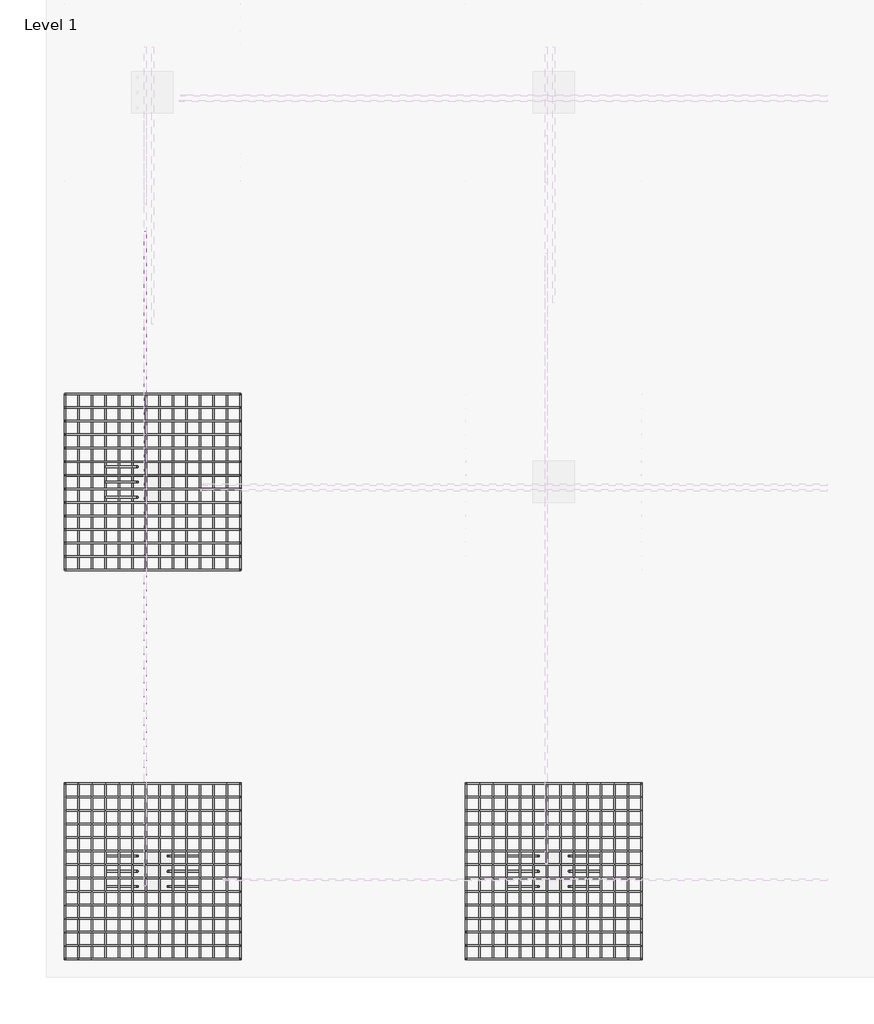
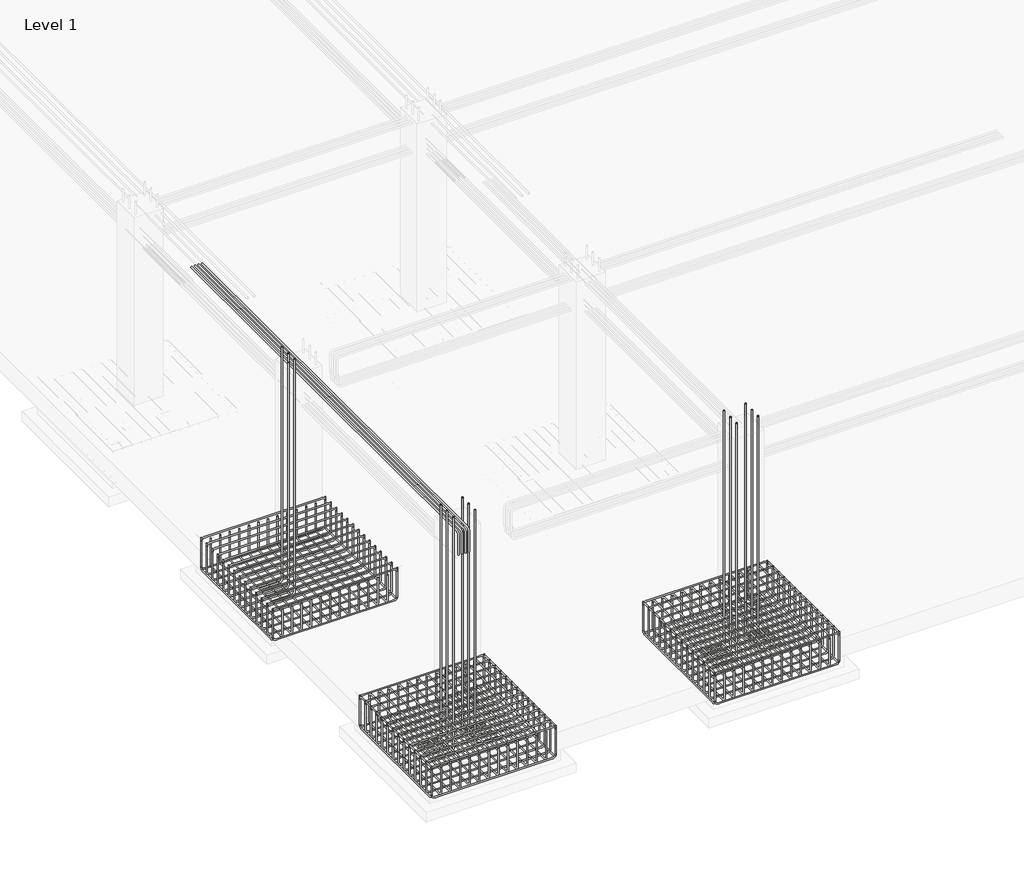
# One storey, part 3 of 17: 18 reinforcing bars.
"""IFC4 building model written with IfcOpenShell, lengths in millimetres."""

from ifc_helpers import new_model, si_unit, point, frame, origin, place, context, project, spatial, polyline, circle_curve, trimmed, segment, composite_curve, source, transform, mapped, element, save
from ifc_brep_helpers import swept_disk

model = new_model("IFC4")

# Units and contexts
model_context = context("Model", 3, world=origin())
ifc_project = project(units=[si_unit("LENGTHUNIT", "METRE", prefix="MILLI")], contexts=[model_context])

# Site, building, storey
site = spatial("IfcSite", under=ifc_project)
building = spatial("IfcBuilding", under=site)
storey = spatial("IfcBuildingStorey", under=building, Name="Level 1", Elevation=0.0)

# Reinforcing bars
placement = place(None, origin())
reinforcing_bar_shape = source(origin(), model_context, "Body", "SolidModel", [
    swept_disk(composite_curve([segment(polyline([(-13686.3632003, 636.009457, -40.0), (-13686.3632003, 636.009457, -504.0)]), True, "CONTINUOUS"), segment(trimmed(circle_curve(frame((-13638.3632003, 636.009457, -504.0), z_axis=(0.0, -1.0, 0.0), x_axis=(-48.0, 0.0, 0.0)), 48.0), [point((-13686.3632003, 636.009457, -504.0))], [point((-13638.3632003, 636.009457, -552.0))], True, "CARTESIAN"), True, "CONTINUOUS"), segment(polyline([(-13638.3632003, 636.009457, -552.0), (-11830.3632003, 636.009457, -552.0)]), True, "CONTINUOUS"), segment(trimmed(circle_curve(frame((-11830.3632003, 636.009457, -504.0), z_axis=(0.0, -1.0, 0.0), x_axis=(0.0, 0.0, -48.0)), 48.0), [point((-11830.3632003, 636.009457, -552.0))], [point((-11782.3632003, 636.009457, -504.0))], True, "CARTESIAN"), True, "CONTINUOUS"), segment(polyline([(-11782.3632003, 636.009457, -504.0), (-11782.3632003, 636.009457, -40.0)]), True, "CONTINUOUS")], self_intersect=False), 8.0),
])
element("IfcReinforcingBar", 1, at=placement, inside=storey, context=model_context, shape_type="MappedRepresentation", body=[
    mapped(reinforcing_bar_shape, transform((0.0, 0.0, 0.0), x_axis=(1.0, 0.0, 0.0), y_axis=(0.0, 1.0, 0.0), z_axis=(0.0, 0.0, 1.0))),
    mapped(reinforcing_bar_shape, transform((0.0, -146.4615385, 0.0), x_axis=(1.0, 0.0, 0.0), y_axis=(0.0, 1.0, 0.0), z_axis=(0.0, 0.0, 1.0))),
    mapped(reinforcing_bar_shape, transform((0.0, -292.9230769, 0.0), x_axis=(1.0, 0.0, 0.0), y_axis=(0.0, 1.0, 0.0), z_axis=(0.0, 0.0, 1.0))),
    mapped(reinforcing_bar_shape, transform((0.0, -439.3846154, 0.0), x_axis=(1.0, 0.0, 0.0), y_axis=(0.0, 1.0, 0.0), z_axis=(0.0, 0.0, 1.0))),
    mapped(reinforcing_bar_shape, transform((0.0, -585.8461538, 0.0), x_axis=(1.0, 0.0, 0.0), y_axis=(0.0, 1.0, 0.0), z_axis=(0.0, 0.0, 1.0))),
    mapped(reinforcing_bar_shape, transform((0.0, -732.3076923, 0.0), x_axis=(1.0, 0.0, 0.0), y_axis=(0.0, 1.0, 0.0), z_axis=(0.0, 0.0, 1.0))),
    mapped(reinforcing_bar_shape, transform((0.0, -878.7692308, 0.0), x_axis=(1.0, 0.0, 0.0), y_axis=(0.0, 1.0, 0.0), z_axis=(0.0, 0.0, 1.0))),
    mapped(reinforcing_bar_shape, transform((0.0, -1025.2307692, 0.0), x_axis=(1.0, 0.0, 0.0), y_axis=(0.0, 1.0, 0.0), z_axis=(0.0, 0.0, 1.0))),
    mapped(reinforcing_bar_shape, transform((0.0, -1171.6923077, 0.0), x_axis=(1.0, 0.0, 0.0), y_axis=(0.0, 1.0, 0.0), z_axis=(0.0, 0.0, 1.0))),
    mapped(reinforcing_bar_shape, transform((0.0, -1318.1538462, 0.0), x_axis=(1.0, 0.0, 0.0), y_axis=(0.0, 1.0, 0.0), z_axis=(0.0, 0.0, 1.0))),
    mapped(reinforcing_bar_shape, transform((0.0, -1464.6153846, 0.0), x_axis=(1.0, 0.0, 0.0), y_axis=(0.0, 1.0, 0.0), z_axis=(0.0, 0.0, 1.0))),
    mapped(reinforcing_bar_shape, transform((0.0, -1611.0769231, 0.0), x_axis=(1.0, 0.0, 0.0), y_axis=(0.0, 1.0, 0.0), z_axis=(0.0, 0.0, 1.0))),
    mapped(reinforcing_bar_shape, transform((0.0, -1757.5384615, 0.0), x_axis=(1.0, 0.0, 0.0), y_axis=(0.0, 1.0, 0.0), z_axis=(0.0, 0.0, 1.0))),
    mapped(reinforcing_bar_shape, transform((0.0, -1904.0, 0.0), x_axis=(1.0, 0.0, 0.0), y_axis=(0.0, 1.0, 0.0), z_axis=(0.0, 0.0, 1.0))),
])
reinforcing_bar_2_shape = source(origin(), model_context, "Body", "SolidModel", [
    swept_disk(composite_curve([segment(polyline([(-13686.3632003, -1267.990543, -504.0), (-13686.3632003, -1267.990543, -96.0)]), True, "CONTINUOUS"), segment(trimmed(circle_curve(frame((-13638.3632003, -1267.990543, -96.0), z_axis=(0.0, 1.0, 0.0), x_axis=(-48.0, 0.0, 0.0)), 48.0), [point((-13686.3632003, -1267.990543, -96.0))], [point((-13638.3632003, -1267.990543, -48.0))], True, "CARTESIAN"), True, "CONTINUOUS"), segment(polyline([(-13638.3632003, -1267.990543, -48.0), (-11830.3632003, -1267.990543, -48.0)]), True, "CONTINUOUS"), segment(trimmed(circle_curve(frame((-11830.3632003, -1267.990543, -96.0), z_axis=(0.0, 1.0, 0.0), x_axis=(0.0, 0.0, 48.0)), 48.0), [point((-11830.3632003, -1267.990543, -48.0))], [point((-11782.3632003, -1267.990543, -96.0))], True, "CARTESIAN"), True, "CONTINUOUS"), segment(polyline([(-11782.3632003, -1267.990543, -96.0), (-11782.3632003, -1267.990543, -504.0)]), True, "CONTINUOUS")], self_intersect=False), 8.0),
])
element("IfcReinforcingBar", 2, at=placement, inside=storey, context=model_context, shape_type="MappedRepresentation", body=[
    mapped(reinforcing_bar_2_shape, transform((0.0, 0.0, 0.0), x_axis=(1.0, 0.0, 0.0), y_axis=(0.0, 1.0, 0.0), z_axis=(0.0, 0.0, 1.0))),
    mapped(reinforcing_bar_2_shape, transform((0.0, 146.4615385, 0.0), x_axis=(1.0, 0.0, 0.0), y_axis=(0.0, 1.0, 0.0), z_axis=(0.0, 0.0, 1.0))),
    mapped(reinforcing_bar_2_shape, transform((0.0, 292.9230769, 0.0), x_axis=(1.0, 0.0, 0.0), y_axis=(0.0, 1.0, 0.0), z_axis=(0.0, 0.0, 1.0))),
    mapped(reinforcing_bar_2_shape, transform((0.0, 439.3846154, 0.0), x_axis=(1.0, 0.0, 0.0), y_axis=(0.0, 1.0, 0.0), z_axis=(0.0, 0.0, 1.0))),
    mapped(reinforcing_bar_2_shape, transform((0.0, 585.8461538, 0.0), x_axis=(1.0, 0.0, 0.0), y_axis=(0.0, 1.0, 0.0), z_axis=(0.0, 0.0, 1.0))),
    mapped(reinforcing_bar_2_shape, transform((0.0, 732.3076923, 0.0), x_axis=(1.0, 0.0, 0.0), y_axis=(0.0, 1.0, 0.0), z_axis=(0.0, 0.0, 1.0))),
    mapped(reinforcing_bar_2_shape, transform((0.0, 878.7692308, 0.0), x_axis=(1.0, 0.0, 0.0), y_axis=(0.0, 1.0, 0.0), z_axis=(0.0, 0.0, 1.0))),
    mapped(reinforcing_bar_2_shape, transform((0.0, 1025.2307692, 0.0), x_axis=(1.0, 0.0, 0.0), y_axis=(0.0, 1.0, 0.0), z_axis=(0.0, 0.0, 1.0))),
    mapped(reinforcing_bar_2_shape, transform((0.0, 1171.6923077, 0.0), x_axis=(1.0, 0.0, 0.0), y_axis=(0.0, 1.0, 0.0), z_axis=(0.0, 0.0, 1.0))),
    mapped(reinforcing_bar_2_shape, transform((0.0, 1318.1538462, 0.0), x_axis=(1.0, 0.0, 0.0), y_axis=(0.0, 1.0, 0.0), z_axis=(0.0, 0.0, 1.0))),
    mapped(reinforcing_bar_2_shape, transform((0.0, 1464.6153846, 0.0), x_axis=(1.0, 0.0, 0.0), y_axis=(0.0, 1.0, 0.0), z_axis=(0.0, 0.0, 1.0))),
    mapped(reinforcing_bar_2_shape, transform((0.0, 1611.0769231, 0.0), x_axis=(1.0, 0.0, 0.0), y_axis=(0.0, 1.0, 0.0), z_axis=(0.0, 0.0, 1.0))),
    mapped(reinforcing_bar_2_shape, transform((0.0, 1757.5384615, 0.0), x_axis=(1.0, 0.0, 0.0), y_axis=(0.0, 1.0, 0.0), z_axis=(0.0, 0.0, 1.0))),
    mapped(reinforcing_bar_2_shape, transform((0.0, 1904.0, 0.0), x_axis=(1.0, 0.0, 0.0), y_axis=(0.0, 1.0, 0.0), z_axis=(0.0, 0.0, 1.0))),
])
reinforcing_bar_3_shape = source(origin(), model_context, "Body", "SolidModel", [
    swept_disk(composite_curve([segment(polyline([(-11782.3632003, 636.009457, -96.0), (-11782.3632003, 636.009457, -504.0)]), True, "CONTINUOUS"), segment(trimmed(circle_curve(frame((-11782.3632003, 588.009457, -504.0), z_axis=(-1.0, 0.0, 0.0), x_axis=(0.0, 48.0, 0.0)), 48.0), [point((-11782.3632003, 636.009457, -504.0))], [point((-11782.3632003, 588.009457, -552.0))], True, "CARTESIAN"), True, "CONTINUOUS"), segment(polyline([(-11782.3632003, 588.009457, -552.0), (-11782.3632003, -1219.990543, -552.0)]), True, "CONTINUOUS"), segment(trimmed(circle_curve(frame((-11782.3632003, -1219.990543, -504.0), z_axis=(-1.0, 0.0, 0.0), x_axis=(0.0, 0.0, -48.0)), 48.0), [point((-11782.3632003, -1219.990543, -552.0))], [point((-11782.3632003, -1267.990543, -504.0))], True, "CARTESIAN"), True, "CONTINUOUS"), segment(polyline([(-11782.3632003, -1267.990543, -504.0), (-11782.3632003, -1267.990543, -96.0)]), True, "CONTINUOUS")], self_intersect=False), 8.0),
])
element("IfcReinforcingBar", 3, at=placement, inside=storey, context=model_context, shape_type="MappedRepresentation", body=[
    mapped(reinforcing_bar_3_shape, transform((0.0, 0.0, 0.0), x_axis=(1.0, 0.0, 0.0), y_axis=(0.0, 1.0, 0.0), z_axis=(0.0, 0.0, 1.0))),
    mapped(reinforcing_bar_3_shape, transform((-146.4615385, 0.0, 0.0), x_axis=(1.0, 0.0, 0.0), y_axis=(0.0, 1.0, 0.0), z_axis=(0.0, 0.0, 1.0))),
    mapped(reinforcing_bar_3_shape, transform((-292.9230769, 0.0, 0.0), x_axis=(1.0, 0.0, 0.0), y_axis=(0.0, 1.0, 0.0), z_axis=(0.0, 0.0, 1.0))),
    mapped(reinforcing_bar_3_shape, transform((-439.3846154, 0.0, 0.0), x_axis=(1.0, 0.0, 0.0), y_axis=(0.0, 1.0, 0.0), z_axis=(0.0, 0.0, 1.0))),
    mapped(reinforcing_bar_3_shape, transform((-585.8461538, 0.0, 0.0), x_axis=(1.0, 0.0, 0.0), y_axis=(0.0, 1.0, 0.0), z_axis=(0.0, 0.0, 1.0))),
    mapped(reinforcing_bar_3_shape, transform((-732.3076923, 0.0, 0.0), x_axis=(1.0, 0.0, 0.0), y_axis=(0.0, 1.0, 0.0), z_axis=(0.0, 0.0, 1.0))),
    mapped(reinforcing_bar_3_shape, transform((-878.7692308, 0.0, 0.0), x_axis=(1.0, 0.0, 0.0), y_axis=(0.0, 1.0, 0.0), z_axis=(0.0, 0.0, 1.0))),
    mapped(reinforcing_bar_3_shape, transform((-1025.2307692, 0.0, 0.0), x_axis=(1.0, 0.0, 0.0), y_axis=(0.0, 1.0, 0.0), z_axis=(0.0, 0.0, 1.0))),
    mapped(reinforcing_bar_3_shape, transform((-1171.6923077, 0.0, 0.0), x_axis=(1.0, 0.0, 0.0), y_axis=(0.0, 1.0, 0.0), z_axis=(0.0, 0.0, 1.0))),
    mapped(reinforcing_bar_3_shape, transform((-1318.1538462, 0.0, 0.0), x_axis=(1.0, 0.0, 0.0), y_axis=(0.0, 1.0, 0.0), z_axis=(0.0, 0.0, 1.0))),
    mapped(reinforcing_bar_3_shape, transform((-1464.6153846, 0.0, 0.0), x_axis=(1.0, 0.0, 0.0), y_axis=(0.0, 1.0, 0.0), z_axis=(0.0, 0.0, 1.0))),
    mapped(reinforcing_bar_3_shape, transform((-1611.0769231, 0.0, 0.0), x_axis=(1.0, 0.0, 0.0), y_axis=(0.0, 1.0, 0.0), z_axis=(0.0, 0.0, 1.0))),
    mapped(reinforcing_bar_3_shape, transform((-1757.5384615, 0.0, 0.0), x_axis=(1.0, 0.0, 0.0), y_axis=(0.0, 1.0, 0.0), z_axis=(0.0, 0.0, 1.0))),
    mapped(reinforcing_bar_3_shape, transform((-1904.0, 0.0, 0.0), x_axis=(1.0, 0.0, 0.0), y_axis=(0.0, 1.0, 0.0), z_axis=(0.0, 0.0, 1.0))),
])
reinforcing_bar_4_shape = source(origin(), model_context, "Body", "SolidModel", [
    swept_disk(composite_curve([segment(polyline([(-13246.9785849, -150.490543, -550.0), (-12949.8632003, -150.490543, -550.0)]), True, "CONTINUOUS"), segment(trimmed(circle_curve(frame((-12949.8632003, -150.490543, -500.0), z_axis=(0.0, -1.0, 0.0), x_axis=(0.0, 0.0, -50.0)), 50.0), [point((-12949.8632003, -150.490543, -550.0))], [point((-12899.8632003, -150.490543, -500.0))], True, "CARTESIAN"), True, "CONTINUOUS"), segment(polyline([(-12899.8632003, -150.490543, -500.0), (-12899.8632003, -150.490543, 3260.0)]), True, "CONTINUOUS")], self_intersect=False), 10.0),
])
element("IfcReinforcingBar", 4, at=placement, inside=storey, context=model_context, shape_type="MappedRepresentation", body=[
    mapped(reinforcing_bar_4_shape, transform((0.0, 0.0, 0.0), x_axis=(1.0, 0.0, 0.0), y_axis=(0.0, 1.0, 0.0), z_axis=(0.0, 0.0, 1.0))),
    mapped(reinforcing_bar_4_shape, transform((0.0, -165.5, 0.0), x_axis=(1.0, 0.0, 0.0), y_axis=(0.0, 1.0, 0.0), z_axis=(0.0, 0.0, 1.0))),
    mapped(reinforcing_bar_4_shape, transform((0.0, -331.0, 0.0), x_axis=(1.0, 0.0, 0.0), y_axis=(0.0, 1.0, 0.0), z_axis=(0.0, 0.0, 1.0))),
])
reinforcing_bar_5_shape = source(origin(), model_context, "Body", "SolidModel", [
    swept_disk(composite_curve([segment(polyline([(-13686.3632003, -3580.990543, -40.0), (-13686.3632003, -3580.990543, -504.0)]), True, "CONTINUOUS"), segment(trimmed(circle_curve(frame((-13638.3632003, -3580.990543, -504.0), z_axis=(0.0, -1.0, 0.0), x_axis=(-48.0, 0.0, 0.0)), 48.0), [point((-13686.3632003, -3580.990543, -504.0))], [point((-13638.3632003, -3580.990543, -552.0))], True, "CARTESIAN"), True, "CONTINUOUS"), segment(polyline([(-13638.3632003, -3580.990543, -552.0), (-11830.3632003, -3580.990543, -552.0)]), True, "CONTINUOUS"), segment(trimmed(circle_curve(frame((-11830.3632003, -3580.990543, -504.0), z_axis=(0.0, -1.0, 0.0), x_axis=(0.0, 0.0, -48.0)), 48.0), [point((-11830.3632003, -3580.990543, -552.0))], [point((-11782.3632003, -3580.990543, -504.0))], True, "CARTESIAN"), True, "CONTINUOUS"), segment(polyline([(-11782.3632003, -3580.990543, -504.0), (-11782.3632003, -3580.990543, -40.0)]), True, "CONTINUOUS")], self_intersect=False), 8.0),
])
element("IfcReinforcingBar", 5, at=placement, inside=storey, context=model_context, shape_type="MappedRepresentation", body=[
    mapped(reinforcing_bar_5_shape, transform((0.0, 0.0, 0.0), x_axis=(1.0, 0.0, 0.0), y_axis=(0.0, 1.0, 0.0), z_axis=(0.0, 0.0, 1.0))),
    mapped(reinforcing_bar_5_shape, transform((0.0, -146.4615385, 0.0), x_axis=(1.0, 0.0, 0.0), y_axis=(0.0, 1.0, 0.0), z_axis=(0.0, 0.0, 1.0))),
    mapped(reinforcing_bar_5_shape, transform((0.0, -292.9230769, 0.0), x_axis=(1.0, 0.0, 0.0), y_axis=(0.0, 1.0, 0.0), z_axis=(0.0, 0.0, 1.0))),
    mapped(reinforcing_bar_5_shape, transform((0.0, -439.3846154, 0.0), x_axis=(1.0, 0.0, 0.0), y_axis=(0.0, 1.0, 0.0), z_axis=(0.0, 0.0, 1.0))),
    mapped(reinforcing_bar_5_shape, transform((0.0, -585.8461538, 0.0), x_axis=(1.0, 0.0, 0.0), y_axis=(0.0, 1.0, 0.0), z_axis=(0.0, 0.0, 1.0))),
    mapped(reinforcing_bar_5_shape, transform((0.0, -732.3076923, 0.0), x_axis=(1.0, 0.0, 0.0), y_axis=(0.0, 1.0, 0.0), z_axis=(0.0, 0.0, 1.0))),
    mapped(reinforcing_bar_5_shape, transform((0.0, -878.7692308, 0.0), x_axis=(1.0, 0.0, 0.0), y_axis=(0.0, 1.0, 0.0), z_axis=(0.0, 0.0, 1.0))),
    mapped(reinforcing_bar_5_shape, transform((0.0, -1025.2307692, 0.0), x_axis=(1.0, 0.0, 0.0), y_axis=(0.0, 1.0, 0.0), z_axis=(0.0, 0.0, 1.0))),
    mapped(reinforcing_bar_5_shape, transform((0.0, -1171.6923077, 0.0), x_axis=(1.0, 0.0, 0.0), y_axis=(0.0, 1.0, 0.0), z_axis=(0.0, 0.0, 1.0))),
    mapped(reinforcing_bar_5_shape, transform((0.0, -1318.1538462, 0.0), x_axis=(1.0, 0.0, 0.0), y_axis=(0.0, 1.0, 0.0), z_axis=(0.0, 0.0, 1.0))),
    mapped(reinforcing_bar_5_shape, transform((0.0, -1464.6153846, 0.0), x_axis=(1.0, 0.0, 0.0), y_axis=(0.0, 1.0, 0.0), z_axis=(0.0, 0.0, 1.0))),
    mapped(reinforcing_bar_5_shape, transform((0.0, -1611.0769231, 0.0), x_axis=(1.0, 0.0, 0.0), y_axis=(0.0, 1.0, 0.0), z_axis=(0.0, 0.0, 1.0))),
    mapped(reinforcing_bar_5_shape, transform((0.0, -1757.5384615, 0.0), x_axis=(1.0, 0.0, 0.0), y_axis=(0.0, 1.0, 0.0), z_axis=(0.0, 0.0, 1.0))),
    mapped(reinforcing_bar_5_shape, transform((0.0, -1904.0, 0.0), x_axis=(1.0, 0.0, 0.0), y_axis=(0.0, 1.0, 0.0), z_axis=(0.0, 0.0, 1.0))),
])
reinforcing_bar_6_shape = source(origin(), model_context, "Body", "SolidModel", [
    swept_disk(composite_curve([segment(polyline([(-13686.3632003, -5484.990543, -504.0), (-13686.3632003, -5484.990543, -96.0)]), True, "CONTINUOUS"), segment(trimmed(circle_curve(frame((-13638.3632003, -5484.990543, -96.0), z_axis=(0.0, 1.0, 0.0), x_axis=(-48.0, 0.0, 0.0)), 48.0), [point((-13686.3632003, -5484.990543, -96.0))], [point((-13638.3632003, -5484.990543, -48.0))], True, "CARTESIAN"), True, "CONTINUOUS"), segment(polyline([(-13638.3632003, -5484.990543, -48.0), (-11830.3632003, -5484.990543, -48.0)]), True, "CONTINUOUS"), segment(trimmed(circle_curve(frame((-11830.3632003, -5484.990543, -96.0), z_axis=(0.0, 1.0, 0.0), x_axis=(0.0, 0.0, 48.0)), 48.0), [point((-11830.3632003, -5484.990543, -48.0))], [point((-11782.3632003, -5484.990543, -96.0))], True, "CARTESIAN"), True, "CONTINUOUS"), segment(polyline([(-11782.3632003, -5484.990543, -96.0), (-11782.3632003, -5484.990543, -504.0)]), True, "CONTINUOUS")], self_intersect=False), 8.0),
])
element("IfcReinforcingBar", 6, at=placement, inside=storey, context=model_context, shape_type="MappedRepresentation", body=[
    mapped(reinforcing_bar_6_shape, transform((0.0, 0.0, 0.0), x_axis=(1.0, 0.0, 0.0), y_axis=(0.0, 1.0, 0.0), z_axis=(0.0, 0.0, 1.0))),
    mapped(reinforcing_bar_6_shape, transform((0.0, 146.4615385, 0.0), x_axis=(1.0, 0.0, 0.0), y_axis=(0.0, 1.0, 0.0), z_axis=(0.0, 0.0, 1.0))),
    mapped(reinforcing_bar_6_shape, transform((0.0, 292.9230769, 0.0), x_axis=(1.0, 0.0, 0.0), y_axis=(0.0, 1.0, 0.0), z_axis=(0.0, 0.0, 1.0))),
    mapped(reinforcing_bar_6_shape, transform((0.0, 439.3846154, 0.0), x_axis=(1.0, 0.0, 0.0), y_axis=(0.0, 1.0, 0.0), z_axis=(0.0, 0.0, 1.0))),
    mapped(reinforcing_bar_6_shape, transform((0.0, 585.8461538, 0.0), x_axis=(1.0, 0.0, 0.0), y_axis=(0.0, 1.0, 0.0), z_axis=(0.0, 0.0, 1.0))),
    mapped(reinforcing_bar_6_shape, transform((0.0, 732.3076923, 0.0), x_axis=(1.0, 0.0, 0.0), y_axis=(0.0, 1.0, 0.0), z_axis=(0.0, 0.0, 1.0))),
    mapped(reinforcing_bar_6_shape, transform((0.0, 878.7692308, 0.0), x_axis=(1.0, 0.0, 0.0), y_axis=(0.0, 1.0, 0.0), z_axis=(0.0, 0.0, 1.0))),
    mapped(reinforcing_bar_6_shape, transform((0.0, 1025.2307692, 0.0), x_axis=(1.0, 0.0, 0.0), y_axis=(0.0, 1.0, 0.0), z_axis=(0.0, 0.0, 1.0))),
    mapped(reinforcing_bar_6_shape, transform((0.0, 1171.6923077, 0.0), x_axis=(1.0, 0.0, 0.0), y_axis=(0.0, 1.0, 0.0), z_axis=(0.0, 0.0, 1.0))),
    mapped(reinforcing_bar_6_shape, transform((0.0, 1318.1538462, 0.0), x_axis=(1.0, 0.0, 0.0), y_axis=(0.0, 1.0, 0.0), z_axis=(0.0, 0.0, 1.0))),
    mapped(reinforcing_bar_6_shape, transform((0.0, 1464.6153846, 0.0), x_axis=(1.0, 0.0, 0.0), y_axis=(0.0, 1.0, 0.0), z_axis=(0.0, 0.0, 1.0))),
    mapped(reinforcing_bar_6_shape, transform((0.0, 1611.0769231, 0.0), x_axis=(1.0, 0.0, 0.0), y_axis=(0.0, 1.0, 0.0), z_axis=(0.0, 0.0, 1.0))),
    mapped(reinforcing_bar_6_shape, transform((0.0, 1757.5384615, 0.0), x_axis=(1.0, 0.0, 0.0), y_axis=(0.0, 1.0, 0.0), z_axis=(0.0, 0.0, 1.0))),
    mapped(reinforcing_bar_6_shape, transform((0.0, 1904.0, 0.0), x_axis=(1.0, 0.0, 0.0), y_axis=(0.0, 1.0, 0.0), z_axis=(0.0, 0.0, 1.0))),
])
reinforcing_bar_7_shape = source(origin(), model_context, "Body", "SolidModel", [
    swept_disk(composite_curve([segment(polyline([(-11782.3632003, -3580.990543, -96.0), (-11782.3632003, -3580.990543, -504.0)]), True, "CONTINUOUS"), segment(trimmed(circle_curve(frame((-11782.3632003, -3628.990543, -504.0), z_axis=(-1.0, 0.0, 0.0), x_axis=(0.0, 48.0, 0.0)), 48.0), [point((-11782.3632003, -3580.990543, -504.0))], [point((-11782.3632003, -3628.990543, -552.0))], True, "CARTESIAN"), True, "CONTINUOUS"), segment(polyline([(-11782.3632003, -3628.990543, -552.0), (-11782.3632003, -5436.990543, -552.0)]), True, "CONTINUOUS"), segment(trimmed(circle_curve(frame((-11782.3632003, -5436.990543, -504.0), z_axis=(-1.0, 0.0, 0.0), x_axis=(0.0, 0.0, -48.0)), 48.0), [point((-11782.3632003, -5436.990543, -552.0))], [point((-11782.3632003, -5484.990543, -504.0))], True, "CARTESIAN"), True, "CONTINUOUS"), segment(polyline([(-11782.3632003, -5484.990543, -504.0), (-11782.3632003, -5484.990543, -96.0)]), True, "CONTINUOUS")], self_intersect=False), 8.0),
])
element("IfcReinforcingBar", 7, at=placement, inside=storey, context=model_context, shape_type="MappedRepresentation", body=[
    mapped(reinforcing_bar_7_shape, transform((0.0, 0.0, 0.0), x_axis=(1.0, 0.0, 0.0), y_axis=(0.0, 1.0, 0.0), z_axis=(0.0, 0.0, 1.0))),
    mapped(reinforcing_bar_7_shape, transform((-146.4615385, 0.0, 0.0), x_axis=(1.0, 0.0, 0.0), y_axis=(0.0, 1.0, 0.0), z_axis=(0.0, 0.0, 1.0))),
    mapped(reinforcing_bar_7_shape, transform((-292.9230769, 0.0, 0.0), x_axis=(1.0, 0.0, 0.0), y_axis=(0.0, 1.0, 0.0), z_axis=(0.0, 0.0, 1.0))),
    mapped(reinforcing_bar_7_shape, transform((-439.3846154, 0.0, 0.0), x_axis=(1.0, 0.0, 0.0), y_axis=(0.0, 1.0, 0.0), z_axis=(0.0, 0.0, 1.0))),
    mapped(reinforcing_bar_7_shape, transform((-585.8461538, 0.0, 0.0), x_axis=(1.0, 0.0, 0.0), y_axis=(0.0, 1.0, 0.0), z_axis=(0.0, 0.0, 1.0))),
    mapped(reinforcing_bar_7_shape, transform((-732.3076923, 0.0, 0.0), x_axis=(1.0, 0.0, 0.0), y_axis=(0.0, 1.0, 0.0), z_axis=(0.0, 0.0, 1.0))),
    mapped(reinforcing_bar_7_shape, transform((-878.7692308, 0.0, 0.0), x_axis=(1.0, 0.0, 0.0), y_axis=(0.0, 1.0, 0.0), z_axis=(0.0, 0.0, 1.0))),
    mapped(reinforcing_bar_7_shape, transform((-1025.2307692, 0.0, 0.0), x_axis=(1.0, 0.0, 0.0), y_axis=(0.0, 1.0, 0.0), z_axis=(0.0, 0.0, 1.0))),
    mapped(reinforcing_bar_7_shape, transform((-1171.6923077, 0.0, 0.0), x_axis=(1.0, 0.0, 0.0), y_axis=(0.0, 1.0, 0.0), z_axis=(0.0, 0.0, 1.0))),
    mapped(reinforcing_bar_7_shape, transform((-1318.1538462, 0.0, 0.0), x_axis=(1.0, 0.0, 0.0), y_axis=(0.0, 1.0, 0.0), z_axis=(0.0, 0.0, 1.0))),
    mapped(reinforcing_bar_7_shape, transform((-1464.6153846, 0.0, 0.0), x_axis=(1.0, 0.0, 0.0), y_axis=(0.0, 1.0, 0.0), z_axis=(0.0, 0.0, 1.0))),
    mapped(reinforcing_bar_7_shape, transform((-1611.0769231, 0.0, 0.0), x_axis=(1.0, 0.0, 0.0), y_axis=(0.0, 1.0, 0.0), z_axis=(0.0, 0.0, 1.0))),
    mapped(reinforcing_bar_7_shape, transform((-1757.5384615, 0.0, 0.0), x_axis=(1.0, 0.0, 0.0), y_axis=(0.0, 1.0, 0.0), z_axis=(0.0, 0.0, 1.0))),
    mapped(reinforcing_bar_7_shape, transform((-1904.0, 0.0, 0.0), x_axis=(1.0, 0.0, 0.0), y_axis=(0.0, 1.0, 0.0), z_axis=(0.0, 0.0, 1.0))),
])
reinforcing_bar_8_shape = source(origin(), model_context, "Body", "SolidModel", [
    swept_disk(composite_curve([segment(polyline([(-13686.3632003, -3580.990543, -504.0), (-13686.3632003, -3580.990543, -96.0)]), True, "CONTINUOUS"), segment(trimmed(circle_curve(frame((-13686.3632003, -3628.990543, -96.0), z_axis=(1.0, 0.0, 0.0), x_axis=(0.0, 48.0, 0.0)), 48.0), [point((-13686.3632003, -3580.990543, -96.0))], [point((-13686.3632003, -3628.990543, -48.0))], True, "CARTESIAN"), True, "CONTINUOUS"), segment(polyline([(-13686.3632003, -3628.990543, -48.0), (-13686.3632003, -5436.990543, -48.0)]), True, "CONTINUOUS"), segment(trimmed(circle_curve(frame((-13686.3632003, -5436.990543, -96.0), z_axis=(1.0, 0.0, 0.0), x_axis=(0.0, 0.0, 48.0)), 48.0), [point((-13686.3632003, -5436.990543, -48.0))], [point((-13686.3632003, -5484.990543, -96.0))], True, "CARTESIAN"), True, "CONTINUOUS"), segment(polyline([(-13686.3632003, -5484.990543, -96.0), (-13686.3632003, -5484.990543, -504.0)]), True, "CONTINUOUS")], self_intersect=False), 8.0),
])
element("IfcReinforcingBar", 8, at=placement, inside=storey, context=model_context, shape_type="MappedRepresentation", body=[
    mapped(reinforcing_bar_8_shape, transform((0.0, 0.0, 0.0), x_axis=(1.0, 0.0, 0.0), y_axis=(0.0, 1.0, 0.0), z_axis=(0.0, 0.0, 1.0))),
    mapped(reinforcing_bar_8_shape, transform((146.4615385, 0.0, 0.0), x_axis=(1.0, 0.0, 0.0), y_axis=(0.0, 1.0, 0.0), z_axis=(0.0, 0.0, 1.0))),
    mapped(reinforcing_bar_8_shape, transform((292.9230769, 0.0, 0.0), x_axis=(1.0, 0.0, 0.0), y_axis=(0.0, 1.0, 0.0), z_axis=(0.0, 0.0, 1.0))),
    mapped(reinforcing_bar_8_shape, transform((439.3846154, 0.0, 0.0), x_axis=(1.0, 0.0, 0.0), y_axis=(0.0, 1.0, 0.0), z_axis=(0.0, 0.0, 1.0))),
    mapped(reinforcing_bar_8_shape, transform((585.8461538, 0.0, 0.0), x_axis=(1.0, 0.0, 0.0), y_axis=(0.0, 1.0, 0.0), z_axis=(0.0, 0.0, 1.0))),
    mapped(reinforcing_bar_8_shape, transform((732.3076923, 0.0, 0.0), x_axis=(1.0, 0.0, 0.0), y_axis=(0.0, 1.0, 0.0), z_axis=(0.0, 0.0, 1.0))),
    mapped(reinforcing_bar_8_shape, transform((878.7692308, 0.0, 0.0), x_axis=(1.0, 0.0, 0.0), y_axis=(0.0, 1.0, 0.0), z_axis=(0.0, 0.0, 1.0))),
    mapped(reinforcing_bar_8_shape, transform((1025.2307692, 0.0, 0.0), x_axis=(1.0, 0.0, 0.0), y_axis=(0.0, 1.0, 0.0), z_axis=(0.0, 0.0, 1.0))),
    mapped(reinforcing_bar_8_shape, transform((1171.6923077, 0.0, 0.0), x_axis=(1.0, 0.0, 0.0), y_axis=(0.0, 1.0, 0.0), z_axis=(0.0, 0.0, 1.0))),
    mapped(reinforcing_bar_8_shape, transform((1318.1538462, 0.0, 0.0), x_axis=(1.0, 0.0, 0.0), y_axis=(0.0, 1.0, 0.0), z_axis=(0.0, 0.0, 1.0))),
    mapped(reinforcing_bar_8_shape, transform((1464.6153846, 0.0, 0.0), x_axis=(1.0, 0.0, 0.0), y_axis=(0.0, 1.0, 0.0), z_axis=(0.0, 0.0, 1.0))),
    mapped(reinforcing_bar_8_shape, transform((1611.0769231, 0.0, 0.0), x_axis=(1.0, 0.0, 0.0), y_axis=(0.0, 1.0, 0.0), z_axis=(0.0, 0.0, 1.0))),
    mapped(reinforcing_bar_8_shape, transform((1757.5384615, 0.0, 0.0), x_axis=(1.0, 0.0, 0.0), y_axis=(0.0, 1.0, 0.0), z_axis=(0.0, 0.0, 1.0))),
    mapped(reinforcing_bar_8_shape, transform((1904.0, 0.0, 0.0), x_axis=(1.0, 0.0, 0.0), y_axis=(0.0, 1.0, 0.0), z_axis=(0.0, 0.0, 1.0))),
])
reinforcing_bar_9_shape = source(origin(), model_context, "Body", "SolidModel", [
    swept_disk(composite_curve([segment(polyline([(-13246.9785849, -4367.490543, -550.0), (-12949.8632003, -4367.490543, -550.0)]), True, "CONTINUOUS"), segment(trimmed(circle_curve(frame((-12949.8632003, -4367.490543, -500.0), z_axis=(0.0, -1.0, 0.0), x_axis=(0.0, 0.0, -50.0)), 50.0), [point((-12949.8632003, -4367.490543, -550.0))], [point((-12899.8632003, -4367.490543, -500.0))], True, "CARTESIAN"), True, "CONTINUOUS"), segment(polyline([(-12899.8632003, -4367.490543, -500.0), (-12899.8632003, -4367.490543, 3260.0)]), True, "CONTINUOUS")], self_intersect=False), 10.0),
])
element("IfcReinforcingBar", 9, at=placement, inside=storey, context=model_context, shape_type="MappedRepresentation", body=[
    mapped(reinforcing_bar_9_shape, transform((0.0, 0.0, 0.0), x_axis=(1.0, 0.0, 0.0), y_axis=(0.0, 1.0, 0.0), z_axis=(0.0, 0.0, 1.0))),
    mapped(reinforcing_bar_9_shape, transform((0.0, -165.5, 0.0), x_axis=(1.0, 0.0, 0.0), y_axis=(0.0, 1.0, 0.0), z_axis=(0.0, 0.0, 1.0))),
    mapped(reinforcing_bar_9_shape, transform((0.0, -331.0, 0.0), x_axis=(1.0, 0.0, 0.0), y_axis=(0.0, 1.0, 0.0), z_axis=(0.0, 0.0, 1.0))),
])
reinforcing_bar_10_shape = source(origin(), model_context, "Body", "SolidModel", [
    swept_disk(composite_curve([segment(polyline([(-12221.7478157, -4698.490543, -550.0), (-12518.8632003, -4698.490543, -550.0)]), True, "CONTINUOUS"), segment(trimmed(circle_curve(frame((-12518.8632003, -4698.490543, -500.0), z_axis=(0.0, 1.0, 0.0), x_axis=(0.0, 0.0, -50.0)), 50.0), [point((-12518.8632003, -4698.490543, -550.0))], [point((-12568.8632003, -4698.490543, -500.0))], True, "CARTESIAN"), True, "CONTINUOUS"), segment(polyline([(-12568.8632003, -4698.490543, -500.0), (-12568.8632003, -4698.490543, 3260.0)]), True, "CONTINUOUS")], self_intersect=False), 10.0),
])
element("IfcReinforcingBar", 10, at=placement, inside=storey, context=model_context, shape_type="MappedRepresentation", body=[
    mapped(reinforcing_bar_10_shape, transform((0.0, 0.0, 0.0), x_axis=(1.0, 0.0, 0.0), y_axis=(0.0, 1.0, 0.0), z_axis=(0.0, 0.0, 1.0))),
    mapped(reinforcing_bar_10_shape, transform((0.0, 165.5, 0.0), x_axis=(1.0, 0.0, 0.0), y_axis=(0.0, 1.0, 0.0), z_axis=(0.0, 0.0, 1.0))),
    mapped(reinforcing_bar_10_shape, transform((0.0, 331.0, 0.0), x_axis=(1.0, 0.0, 0.0), y_axis=(0.0, 1.0, 0.0), z_axis=(0.0, 0.0, 1.0))),
])
reinforcing_bar_11_shape = source(origin(), model_context, "Body", "SolidModel", [
    swept_disk(composite_curve([segment(polyline([(-9341.3632003, -3580.990543, -40.0), (-9341.3632003, -3580.990543, -504.0)]), True, "CONTINUOUS"), segment(trimmed(circle_curve(frame((-9293.3632003, -3580.990543, -504.0), z_axis=(0.0, -1.0, 0.0), x_axis=(-48.0, 0.0, 0.0)), 48.0), [point((-9341.3632003, -3580.990543, -504.0))], [point((-9293.3632003, -3580.990543, -552.0))], True, "CARTESIAN"), True, "CONTINUOUS"), segment(polyline([(-9293.3632003, -3580.990543, -552.0), (-7485.3632003, -3580.990543, -552.0)]), True, "CONTINUOUS"), segment(trimmed(circle_curve(frame((-7485.3632003, -3580.990543, -504.0), z_axis=(0.0, -1.0, 0.0), x_axis=(0.0, 0.0, -48.0)), 48.0), [point((-7485.3632003, -3580.990543, -552.0))], [point((-7437.3632003, -3580.990543, -504.0))], True, "CARTESIAN"), True, "CONTINUOUS"), segment(polyline([(-7437.3632003, -3580.990543, -504.0), (-7437.3632003, -3580.990543, -40.0)]), True, "CONTINUOUS")], self_intersect=False), 8.0),
])
element("IfcReinforcingBar", 11, at=placement, inside=storey, context=model_context, shape_type="MappedRepresentation", body=[
    mapped(reinforcing_bar_11_shape, transform((0.0, 0.0, 0.0), x_axis=(1.0, 0.0, 0.0), y_axis=(0.0, 1.0, 0.0), z_axis=(0.0, 0.0, 1.0))),
    mapped(reinforcing_bar_11_shape, transform((0.0, -146.4615385, 0.0), x_axis=(1.0, 0.0, 0.0), y_axis=(0.0, 1.0, 0.0), z_axis=(0.0, 0.0, 1.0))),
    mapped(reinforcing_bar_11_shape, transform((0.0, -292.9230769, 0.0), x_axis=(1.0, 0.0, 0.0), y_axis=(0.0, 1.0, 0.0), z_axis=(0.0, 0.0, 1.0))),
    mapped(reinforcing_bar_11_shape, transform((0.0, -439.3846154, 0.0), x_axis=(1.0, 0.0, 0.0), y_axis=(0.0, 1.0, 0.0), z_axis=(0.0, 0.0, 1.0))),
    mapped(reinforcing_bar_11_shape, transform((0.0, -585.8461538, 0.0), x_axis=(1.0, 0.0, 0.0), y_axis=(0.0, 1.0, 0.0), z_axis=(0.0, 0.0, 1.0))),
    mapped(reinforcing_bar_11_shape, transform((0.0, -732.3076923, 0.0), x_axis=(1.0, 0.0, 0.0), y_axis=(0.0, 1.0, 0.0), z_axis=(0.0, 0.0, 1.0))),
    mapped(reinforcing_bar_11_shape, transform((0.0, -878.7692308, 0.0), x_axis=(1.0, 0.0, 0.0), y_axis=(0.0, 1.0, 0.0), z_axis=(0.0, 0.0, 1.0))),
    mapped(reinforcing_bar_11_shape, transform((0.0, -1025.2307692, 0.0), x_axis=(1.0, 0.0, 0.0), y_axis=(0.0, 1.0, 0.0), z_axis=(0.0, 0.0, 1.0))),
    mapped(reinforcing_bar_11_shape, transform((0.0, -1171.6923077, 0.0), x_axis=(1.0, 0.0, 0.0), y_axis=(0.0, 1.0, 0.0), z_axis=(0.0, 0.0, 1.0))),
    mapped(reinforcing_bar_11_shape, transform((0.0, -1318.1538462, 0.0), x_axis=(1.0, 0.0, 0.0), y_axis=(0.0, 1.0, 0.0), z_axis=(0.0, 0.0, 1.0))),
    mapped(reinforcing_bar_11_shape, transform((0.0, -1464.6153846, 0.0), x_axis=(1.0, 0.0, 0.0), y_axis=(0.0, 1.0, 0.0), z_axis=(0.0, 0.0, 1.0))),
    mapped(reinforcing_bar_11_shape, transform((0.0, -1611.0769231, 0.0), x_axis=(1.0, 0.0, 0.0), y_axis=(0.0, 1.0, 0.0), z_axis=(0.0, 0.0, 1.0))),
    mapped(reinforcing_bar_11_shape, transform((0.0, -1757.5384615, 0.0), x_axis=(1.0, 0.0, 0.0), y_axis=(0.0, 1.0, 0.0), z_axis=(0.0, 0.0, 1.0))),
    mapped(reinforcing_bar_11_shape, transform((0.0, -1904.0, 0.0), x_axis=(1.0, 0.0, 0.0), y_axis=(0.0, 1.0, 0.0), z_axis=(0.0, 0.0, 1.0))),
])
reinforcing_bar_12_shape = source(origin(), model_context, "Body", "SolidModel", [
    swept_disk(composite_curve([segment(polyline([(-9341.3632003, -5484.990543, -504.0), (-9341.3632003, -5484.990543, -96.0)]), True, "CONTINUOUS"), segment(trimmed(circle_curve(frame((-9293.3632003, -5484.990543, -96.0), z_axis=(0.0, 1.0, 0.0), x_axis=(-48.0, 0.0, 0.0)), 48.0), [point((-9341.3632003, -5484.990543, -96.0))], [point((-9293.3632003, -5484.990543, -48.0))], True, "CARTESIAN"), True, "CONTINUOUS"), segment(polyline([(-9293.3632003, -5484.990543, -48.0), (-7485.3632003, -5484.990543, -48.0)]), True, "CONTINUOUS"), segment(trimmed(circle_curve(frame((-7485.3632003, -5484.990543, -96.0), z_axis=(0.0, 1.0, 0.0), x_axis=(0.0, 0.0, 48.0)), 48.0), [point((-7485.3632003, -5484.990543, -48.0))], [point((-7437.3632003, -5484.990543, -96.0))], True, "CARTESIAN"), True, "CONTINUOUS"), segment(polyline([(-7437.3632003, -5484.990543, -96.0), (-7437.3632003, -5484.990543, -504.0)]), True, "CONTINUOUS")], self_intersect=False), 8.0),
])
element("IfcReinforcingBar", 12, at=placement, inside=storey, context=model_context, shape_type="MappedRepresentation", body=[
    mapped(reinforcing_bar_12_shape, transform((0.0, 0.0, 0.0), x_axis=(1.0, 0.0, 0.0), y_axis=(0.0, 1.0, 0.0), z_axis=(0.0, 0.0, 1.0))),
    mapped(reinforcing_bar_12_shape, transform((0.0, 146.4615385, 0.0), x_axis=(1.0, 0.0, 0.0), y_axis=(0.0, 1.0, 0.0), z_axis=(0.0, 0.0, 1.0))),
    mapped(reinforcing_bar_12_shape, transform((0.0, 292.9230769, 0.0), x_axis=(1.0, 0.0, 0.0), y_axis=(0.0, 1.0, 0.0), z_axis=(0.0, 0.0, 1.0))),
    mapped(reinforcing_bar_12_shape, transform((0.0, 439.3846154, 0.0), x_axis=(1.0, 0.0, 0.0), y_axis=(0.0, 1.0, 0.0), z_axis=(0.0, 0.0, 1.0))),
    mapped(reinforcing_bar_12_shape, transform((0.0, 585.8461538, 0.0), x_axis=(1.0, 0.0, 0.0), y_axis=(0.0, 1.0, 0.0), z_axis=(0.0, 0.0, 1.0))),
    mapped(reinforcing_bar_12_shape, transform((0.0, 732.3076923, 0.0), x_axis=(1.0, 0.0, 0.0), y_axis=(0.0, 1.0, 0.0), z_axis=(0.0, 0.0, 1.0))),
    mapped(reinforcing_bar_12_shape, transform((0.0, 878.7692308, 0.0), x_axis=(1.0, 0.0, 0.0), y_axis=(0.0, 1.0, 0.0), z_axis=(0.0, 0.0, 1.0))),
    mapped(reinforcing_bar_12_shape, transform((0.0, 1025.2307692, 0.0), x_axis=(1.0, 0.0, 0.0), y_axis=(0.0, 1.0, 0.0), z_axis=(0.0, 0.0, 1.0))),
    mapped(reinforcing_bar_12_shape, transform((0.0, 1171.6923077, 0.0), x_axis=(1.0, 0.0, 0.0), y_axis=(0.0, 1.0, 0.0), z_axis=(0.0, 0.0, 1.0))),
    mapped(reinforcing_bar_12_shape, transform((0.0, 1318.1538462, 0.0), x_axis=(1.0, 0.0, 0.0), y_axis=(0.0, 1.0, 0.0), z_axis=(0.0, 0.0, 1.0))),
    mapped(reinforcing_bar_12_shape, transform((0.0, 1464.6153846, 0.0), x_axis=(1.0, 0.0, 0.0), y_axis=(0.0, 1.0, 0.0), z_axis=(0.0, 0.0, 1.0))),
    mapped(reinforcing_bar_12_shape, transform((0.0, 1611.0769231, 0.0), x_axis=(1.0, 0.0, 0.0), y_axis=(0.0, 1.0, 0.0), z_axis=(0.0, 0.0, 1.0))),
    mapped(reinforcing_bar_12_shape, transform((0.0, 1757.5384615, 0.0), x_axis=(1.0, 0.0, 0.0), y_axis=(0.0, 1.0, 0.0), z_axis=(0.0, 0.0, 1.0))),
    mapped(reinforcing_bar_12_shape, transform((0.0, 1904.0, 0.0), x_axis=(1.0, 0.0, 0.0), y_axis=(0.0, 1.0, 0.0), z_axis=(0.0, 0.0, 1.0))),
])
reinforcing_bar_13_shape = source(origin(), model_context, "Body", "SolidModel", [
    swept_disk(composite_curve([segment(polyline([(-7437.3632003, -3580.990543, -96.0), (-7437.3632003, -3580.990543, -504.0)]), True, "CONTINUOUS"), segment(trimmed(circle_curve(frame((-7437.3632003, -3628.990543, -504.0), z_axis=(-1.0, 0.0, 0.0), x_axis=(0.0, 48.0, 0.0)), 48.0), [point((-7437.3632003, -3580.990543, -504.0))], [point((-7437.3632003, -3628.990543, -552.0))], True, "CARTESIAN"), True, "CONTINUOUS"), segment(polyline([(-7437.3632003, -3628.990543, -552.0), (-7437.3632003, -5436.990543, -552.0)]), True, "CONTINUOUS"), segment(trimmed(circle_curve(frame((-7437.3632003, -5436.990543, -504.0), z_axis=(-1.0, 0.0, 0.0), x_axis=(0.0, 0.0, -48.0)), 48.0), [point((-7437.3632003, -5436.990543, -552.0))], [point((-7437.3632003, -5484.990543, -504.0))], True, "CARTESIAN"), True, "CONTINUOUS"), segment(polyline([(-7437.3632003, -5484.990543, -504.0), (-7437.3632003, -5484.990543, -96.0)]), True, "CONTINUOUS")], self_intersect=False), 8.0),
])
element("IfcReinforcingBar", 13, at=placement, inside=storey, context=model_context, shape_type="MappedRepresentation", body=[
    mapped(reinforcing_bar_13_shape, transform((0.0, 0.0, 0.0), x_axis=(1.0, 0.0, 0.0), y_axis=(0.0, 1.0, 0.0), z_axis=(0.0, 0.0, 1.0))),
    mapped(reinforcing_bar_13_shape, transform((-146.4615385, 0.0, 0.0), x_axis=(1.0, 0.0, 0.0), y_axis=(0.0, 1.0, 0.0), z_axis=(0.0, 0.0, 1.0))),
    mapped(reinforcing_bar_13_shape, transform((-292.9230769, 0.0, 0.0), x_axis=(1.0, 0.0, 0.0), y_axis=(0.0, 1.0, 0.0), z_axis=(0.0, 0.0, 1.0))),
    mapped(reinforcing_bar_13_shape, transform((-439.3846154, 0.0, 0.0), x_axis=(1.0, 0.0, 0.0), y_axis=(0.0, 1.0, 0.0), z_axis=(0.0, 0.0, 1.0))),
    mapped(reinforcing_bar_13_shape, transform((-585.8461538, 0.0, 0.0), x_axis=(1.0, 0.0, 0.0), y_axis=(0.0, 1.0, 0.0), z_axis=(0.0, 0.0, 1.0))),
    mapped(reinforcing_bar_13_shape, transform((-732.3076923, 0.0, 0.0), x_axis=(1.0, 0.0, 0.0), y_axis=(0.0, 1.0, 0.0), z_axis=(0.0, 0.0, 1.0))),
    mapped(reinforcing_bar_13_shape, transform((-878.7692308, 0.0, 0.0), x_axis=(1.0, 0.0, 0.0), y_axis=(0.0, 1.0, 0.0), z_axis=(0.0, 0.0, 1.0))),
    mapped(reinforcing_bar_13_shape, transform((-1025.2307692, 0.0, 0.0), x_axis=(1.0, 0.0, 0.0), y_axis=(0.0, 1.0, 0.0), z_axis=(0.0, 0.0, 1.0))),
    mapped(reinforcing_bar_13_shape, transform((-1171.6923077, 0.0, 0.0), x_axis=(1.0, 0.0, 0.0), y_axis=(0.0, 1.0, 0.0), z_axis=(0.0, 0.0, 1.0))),
    mapped(reinforcing_bar_13_shape, transform((-1318.1538462, 0.0, 0.0), x_axis=(1.0, 0.0, 0.0), y_axis=(0.0, 1.0, 0.0), z_axis=(0.0, 0.0, 1.0))),
    mapped(reinforcing_bar_13_shape, transform((-1464.6153846, 0.0, 0.0), x_axis=(1.0, 0.0, 0.0), y_axis=(0.0, 1.0, 0.0), z_axis=(0.0, 0.0, 1.0))),
    mapped(reinforcing_bar_13_shape, transform((-1611.0769231, 0.0, 0.0), x_axis=(1.0, 0.0, 0.0), y_axis=(0.0, 1.0, 0.0), z_axis=(0.0, 0.0, 1.0))),
    mapped(reinforcing_bar_13_shape, transform((-1757.5384615, 0.0, 0.0), x_axis=(1.0, 0.0, 0.0), y_axis=(0.0, 1.0, 0.0), z_axis=(0.0, 0.0, 1.0))),
    mapped(reinforcing_bar_13_shape, transform((-1904.0, 0.0, 0.0), x_axis=(1.0, 0.0, 0.0), y_axis=(0.0, 1.0, 0.0), z_axis=(0.0, 0.0, 1.0))),
])
reinforcing_bar_14_shape = source(origin(), model_context, "Body", "SolidModel", [
    swept_disk(composite_curve([segment(polyline([(-9341.3632003, -3580.990543, -504.0), (-9341.3632003, -3580.990543, -96.0)]), True, "CONTINUOUS"), segment(trimmed(circle_curve(frame((-9341.3632003, -3628.990543, -96.0), z_axis=(1.0, 0.0, 0.0), x_axis=(0.0, 48.0, 0.0)), 48.0), [point((-9341.3632003, -3580.990543, -96.0))], [point((-9341.3632003, -3628.990543, -48.0))], True, "CARTESIAN"), True, "CONTINUOUS"), segment(polyline([(-9341.3632003, -3628.990543, -48.0), (-9341.3632003, -5436.990543, -48.0)]), True, "CONTINUOUS"), segment(trimmed(circle_curve(frame((-9341.3632003, -5436.990543, -96.0), z_axis=(1.0, 0.0, 0.0), x_axis=(0.0, 0.0, 48.0)), 48.0), [point((-9341.3632003, -5436.990543, -48.0))], [point((-9341.3632003, -5484.990543, -96.0))], True, "CARTESIAN"), True, "CONTINUOUS"), segment(polyline([(-9341.3632003, -5484.990543, -96.0), (-9341.3632003, -5484.990543, -504.0)]), True, "CONTINUOUS")], self_intersect=False), 8.0),
])
element("IfcReinforcingBar", 14, at=placement, inside=storey, context=model_context, shape_type="MappedRepresentation", body=[
    mapped(reinforcing_bar_14_shape, transform((0.0, 0.0, 0.0), x_axis=(1.0, 0.0, 0.0), y_axis=(0.0, 1.0, 0.0), z_axis=(0.0, 0.0, 1.0))),
    mapped(reinforcing_bar_14_shape, transform((146.4615385, 0.0, 0.0), x_axis=(1.0, 0.0, 0.0), y_axis=(0.0, 1.0, 0.0), z_axis=(0.0, 0.0, 1.0))),
    mapped(reinforcing_bar_14_shape, transform((292.9230769, 0.0, 0.0), x_axis=(1.0, 0.0, 0.0), y_axis=(0.0, 1.0, 0.0), z_axis=(0.0, 0.0, 1.0))),
    mapped(reinforcing_bar_14_shape, transform((439.3846154, 0.0, 0.0), x_axis=(1.0, 0.0, 0.0), y_axis=(0.0, 1.0, 0.0), z_axis=(0.0, 0.0, 1.0))),
    mapped(reinforcing_bar_14_shape, transform((585.8461538, 0.0, 0.0), x_axis=(1.0, 0.0, 0.0), y_axis=(0.0, 1.0, 0.0), z_axis=(0.0, 0.0, 1.0))),
    mapped(reinforcing_bar_14_shape, transform((732.3076923, 0.0, 0.0), x_axis=(1.0, 0.0, 0.0), y_axis=(0.0, 1.0, 0.0), z_axis=(0.0, 0.0, 1.0))),
    mapped(reinforcing_bar_14_shape, transform((878.7692308, 0.0, 0.0), x_axis=(1.0, 0.0, 0.0), y_axis=(0.0, 1.0, 0.0), z_axis=(0.0, 0.0, 1.0))),
    mapped(reinforcing_bar_14_shape, transform((1025.2307692, 0.0, 0.0), x_axis=(1.0, 0.0, 0.0), y_axis=(0.0, 1.0, 0.0), z_axis=(0.0, 0.0, 1.0))),
    mapped(reinforcing_bar_14_shape, transform((1171.6923077, 0.0, 0.0), x_axis=(1.0, 0.0, 0.0), y_axis=(0.0, 1.0, 0.0), z_axis=(0.0, 0.0, 1.0))),
    mapped(reinforcing_bar_14_shape, transform((1318.1538462, 0.0, 0.0), x_axis=(1.0, 0.0, 0.0), y_axis=(0.0, 1.0, 0.0), z_axis=(0.0, 0.0, 1.0))),
    mapped(reinforcing_bar_14_shape, transform((1464.6153846, 0.0, 0.0), x_axis=(1.0, 0.0, 0.0), y_axis=(0.0, 1.0, 0.0), z_axis=(0.0, 0.0, 1.0))),
    mapped(reinforcing_bar_14_shape, transform((1611.0769231, 0.0, 0.0), x_axis=(1.0, 0.0, 0.0), y_axis=(0.0, 1.0, 0.0), z_axis=(0.0, 0.0, 1.0))),
    mapped(reinforcing_bar_14_shape, transform((1757.5384615, 0.0, 0.0), x_axis=(1.0, 0.0, 0.0), y_axis=(0.0, 1.0, 0.0), z_axis=(0.0, 0.0, 1.0))),
    mapped(reinforcing_bar_14_shape, transform((1904.0, 0.0, 0.0), x_axis=(1.0, 0.0, 0.0), y_axis=(0.0, 1.0, 0.0), z_axis=(0.0, 0.0, 1.0))),
])
reinforcing_bar_15_shape = source(origin(), model_context, "Body", "SolidModel", [
    swept_disk(composite_curve([segment(polyline([(-8901.9785849, -4367.490543, -550.0), (-8604.8632003, -4367.490543, -550.0)]), True, "CONTINUOUS"), segment(trimmed(circle_curve(frame((-8604.8632003, -4367.490543, -500.0), z_axis=(0.0, -1.0, 0.0), x_axis=(0.0, 0.0, -50.0)), 50.0), [point((-8604.8632003, -4367.490543, -550.0))], [point((-8554.8632003, -4367.490543, -500.0))], True, "CARTESIAN"), True, "CONTINUOUS"), segment(polyline([(-8554.8632003, -4367.490543, -500.0), (-8554.8632003, -4367.490543, 3260.0)]), True, "CONTINUOUS")], self_intersect=False), 10.0),
])
element("IfcReinforcingBar", 15, at=placement, inside=storey, context=model_context, shape_type="MappedRepresentation", body=[
    mapped(reinforcing_bar_15_shape, transform((0.0, 0.0, 0.0), x_axis=(1.0, 0.0, 0.0), y_axis=(0.0, 1.0, 0.0), z_axis=(0.0, 0.0, 1.0))),
    mapped(reinforcing_bar_15_shape, transform((0.0, -165.5, 0.0), x_axis=(1.0, 0.0, 0.0), y_axis=(0.0, 1.0, 0.0), z_axis=(0.0, 0.0, 1.0))),
    mapped(reinforcing_bar_15_shape, transform((0.0, -331.0, 0.0), x_axis=(1.0, 0.0, 0.0), y_axis=(0.0, 1.0, 0.0), z_axis=(0.0, 0.0, 1.0))),
])
reinforcing_bar_16_shape = source(origin(), model_context, "Body", "SolidModel", [
    swept_disk(composite_curve([segment(polyline([(-7876.7478157, -4698.490543, -550.0), (-8173.8632003, -4698.490543, -550.0)]), True, "CONTINUOUS"), segment(trimmed(circle_curve(frame((-8173.8632003, -4698.490543, -500.0), z_axis=(0.0, 1.0, 0.0), x_axis=(0.0, 0.0, -50.0)), 50.0), [point((-8173.8632003, -4698.490543, -550.0))], [point((-8223.8632003, -4698.490543, -500.0))], True, "CARTESIAN"), True, "CONTINUOUS"), segment(polyline([(-8223.8632003, -4698.490543, -500.0), (-8223.8632003, -4698.490543, 3260.0)]), True, "CONTINUOUS")], self_intersect=False), 10.0),
])
element("IfcReinforcingBar", 16, at=placement, inside=storey, context=model_context, shape_type="MappedRepresentation", body=[
    mapped(reinforcing_bar_16_shape, transform((0.0, 0.0, 0.0), x_axis=(1.0, 0.0, 0.0), y_axis=(0.0, 1.0, 0.0), z_axis=(0.0, 0.0, 1.0))),
    mapped(reinforcing_bar_16_shape, transform((0.0, 165.5, 0.0), x_axis=(1.0, 0.0, 0.0), y_axis=(0.0, 1.0, 0.0), z_axis=(0.0, 0.0, 1.0))),
    mapped(reinforcing_bar_16_shape, transform((0.0, 331.0, 0.0), x_axis=(1.0, 0.0, 0.0), y_axis=(0.0, 1.0, 0.0), z_axis=(0.0, 0.0, 1.0))),
])
reinforcing_bar_17_shape = source(origin(), model_context, "Body", "SolidModel", [
    swept_disk(composite_curve([segment(polyline([(-12814.3632003, 2401.009457, 2978.0), (-12814.3632003, -4638.490543, 2978.0)]), True, "CONTINUOUS"), segment(trimmed(circle_curve(frame((-12814.3632003, -4638.490543, 2928.0), z_axis=(1.0, 0.0, 0.0), x_axis=(0.0, 0.0, 50.0)), 50.0), [point((-12814.3632003, -4638.490543, 2978.0))], [point((-12814.3632003, -4688.490543, 2928.0))], True, "CARTESIAN"), True, "CONTINUOUS"), segment(polyline([(-12814.3632003, -4688.490543, 2928.0), (-12814.3632003, -4688.490543, 2608.0)]), True, "CONTINUOUS")], self_intersect=False), 10.0),
])
element("IfcReinforcingBar", 17, at=placement, inside=storey, context=model_context, shape_type="MappedRepresentation", body=[
    mapped(reinforcing_bar_17_shape, transform((0.0, 0.0, 0.0), x_axis=(1.0, 0.0, 0.0), y_axis=(0.0, 1.0, 0.0), z_axis=(0.0, 0.0, 1.0))),
    mapped(reinforcing_bar_17_shape, transform((53.3333333, 0.0, 0.0), x_axis=(1.0, 0.0, 0.0), y_axis=(0.0, 1.0, 0.0), z_axis=(0.0, 0.0, 1.0))),
    mapped(reinforcing_bar_17_shape, transform((106.6666667, 0.0, 0.0), x_axis=(1.0, 0.0, 0.0), y_axis=(0.0, 1.0, 0.0), z_axis=(0.0, 0.0, 1.0))),
    mapped(reinforcing_bar_17_shape, transform((160.0, 0.0, 0.0), x_axis=(1.0, 0.0, 0.0), y_axis=(0.0, 1.0, 0.0), z_axis=(0.0, 0.0, 1.0))),
])
reinforcing_bar_18_shape = source(origin(), model_context, "Body", "SolidModel", [
    swept_disk(composite_curve([segment(polyline([(-12814.3632003, 2401.009457, 2978.0), (-12814.3632003, -4638.490543, 2978.0)]), True, "CONTINUOUS"), segment(trimmed(circle_curve(frame((-12814.3632003, -4638.490543, 2928.0), z_axis=(1.0, 0.0, 0.0), x_axis=(0.0, 0.0, 50.0)), 50.0), [point((-12814.3632003, -4638.490543, 2978.0))], [point((-12814.3632003, -4688.490543, 2928.0))], True, "CARTESIAN"), True, "CONTINUOUS"), segment(polyline([(-12814.3632003, -4688.490543, 2928.0), (-12814.3632003, -4688.490543, 2608.0)]), True, "CONTINUOUS")], self_intersect=False), 10.0),
])
element("IfcReinforcingBar", 18, at=placement, inside=storey, context=model_context, shape_type="MappedRepresentation", body=[
    mapped(reinforcing_bar_18_shape, transform((0.0, 0.0, 0.0), x_axis=(1.0, 0.0, 0.0), y_axis=(0.0, 1.0, 0.0), z_axis=(0.0, 0.0, 1.0))),
    mapped(reinforcing_bar_18_shape, transform((53.3333333, 0.0, 0.0), x_axis=(1.0, 0.0, 0.0), y_axis=(0.0, 1.0, 0.0), z_axis=(0.0, 0.0, 1.0))),
    mapped(reinforcing_bar_18_shape, transform((106.6666667, 0.0, 0.0), x_axis=(1.0, 0.0, 0.0), y_axis=(0.0, 1.0, 0.0), z_axis=(0.0, 0.0, 1.0))),
    mapped(reinforcing_bar_18_shape, transform((160.0, 0.0, 0.0), x_axis=(1.0, 0.0, 0.0), y_axis=(0.0, 1.0, 0.0), z_axis=(0.0, 0.0, 1.0))),
])

save(model, "model.ifc")

# Revit data of these elements
# Elements 1, 2, 3, 4, 5, 6, 7, 8, 9, 10, 11, 12, 13, 14, 15, 16, 17, 18 (IfcReinforcingBar)
#   Phase Created = New Construction
